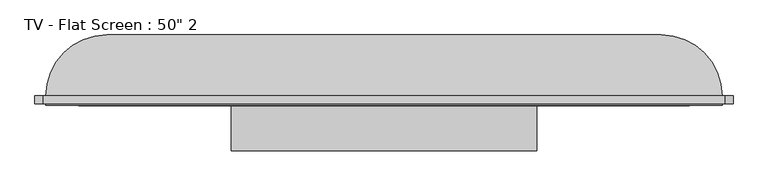
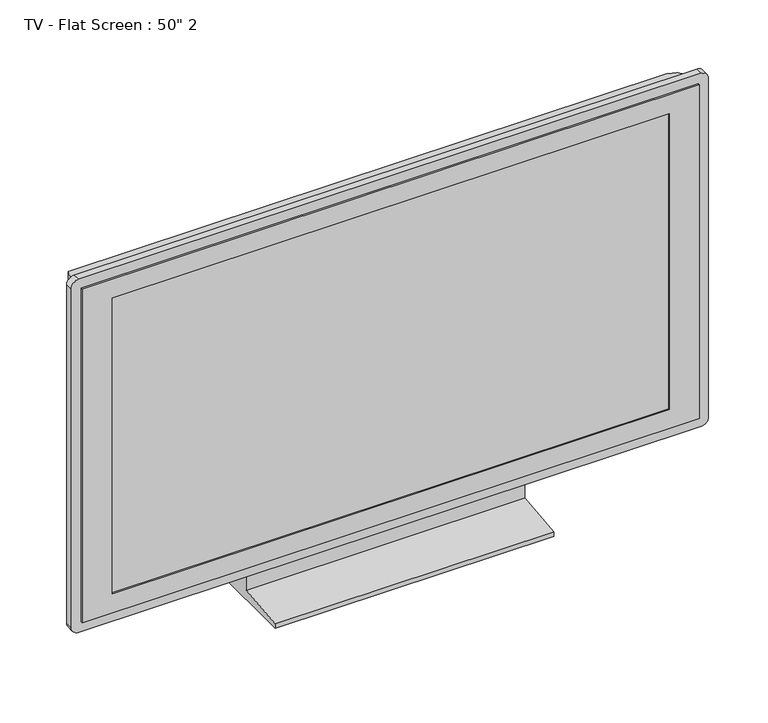
"""IFC4 building model written with IfcOpenShell, lengths in millimetres: furniture geometry."""

from ifc_helpers import new_model, si_unit, point, frame, frame_2d, origin, place, context, project, spatial, polyline, circle_curve, ellipse_curve, trimmed, segment, composite_curve, outline, extrude, faceted_brep, source, transform, mapped, element, save
from ifc_brep_helpers import plane_surface, cylinder_surface, advanced_brep


def furniture_0b81fedb(model_context):
    return source(origin(), model_context, "Body", "SolidModel", [
        advanced_brep(
        [(-617.3827737, -51.4613764, 80.0), (609.4937454, -51.4613764, 80.0), (609.4937454, -51.4613764, 782.6751733), (-617.3827737, -51.4613764, 782.6751733), (499.4937454, 58.5386236, 80.0), (-507.3827737, 58.5386236, 80.0), (-507.3827737, 58.5386236, 672.6751733), (499.4937454, 58.5386236, 672.6751733)],
        [
            (0, 1),
            (1, 2),
            (2, 3),
            (3, 0),
            (4, 5),
            (5, 6),
            (6, 7),
            (7, 4),
            (0, 5, circle_curve(frame((-507.3827737, -51.4613764, 80.0), z_axis=(0.0, 0.0, -1.0), x_axis=(-1.0, 0.0, 0.0)), 110.0)),
            (4, 1, circle_curve(frame((499.4937454, -51.4613764, 80.0), z_axis=(0.0, 0.0, -1.0), x_axis=(1.0, 0.0, 0.0)), 110.0)),
            (7, 2, ellipse_curve(frame((499.4937454, -51.4613764, 672.6751733), z_axis=(0.7071067811865475, 0.0, -0.7071067811865475), x_axis=(0.7071067811865474, 0.0, 0.7071067811865476)), 155.5634919, 110.0)),
            (6, 3, ellipse_curve(frame((-507.3827737, -51.4613764, 672.6751733), z_axis=(0.7071067811865475, 0.0, 0.7071067811865475), x_axis=(-0.7071067811865476, 0.0, 0.7071067811865474)), 155.5634919, 110.0)),
        ],
        [
            plane_surface(frame((-617.3827737, -51.4613764, 782.6751733), z_axis=(0.0, -1.0, 0.0), x_axis=(-1.0, 0.0, 0.0))),
            plane_surface(frame((-617.3827737, 58.5386236, 782.6751733), z_axis=(0.0, 1.0, 0.0), x_axis=(1.0, 0.0, 0.0))),
            plane_surface(frame((-617.3827737, -51.4613764, 80.0), z_axis=(0.0, 0.0, -1.0), x_axis=(0.0, 1.0, 0.0))),
            cylinder_surface(frame((499.4937454, -51.4613764, 80.0), z_axis=(0.0, 0.0, 1.0), x_axis=(1.0, 0.0, 0.0)), 110.0),
            cylinder_surface(frame((609.4937454, -51.4613764, 672.6751733), z_axis=(-1.0, 0.0, 0.0), x_axis=(0.0, 0.0, 1.0)), 110.0),
            cylinder_surface(frame((-507.3827737, -51.4613764, 782.6751733), z_axis=(0.0, 0.0, -1.0), x_axis=(-1.0, 0.0, 0.0)), 110.0),
        ],
        [
            (0, [[1, 2, 3, 4]]),
            (1, [[5, 6, 7, 8]]),
            (2, [[-1, 9, -5, 10]]),
            (3, [[11, -2, -10, -8]]),
            (4, [[-11, -7, 12, -3]]),
            (5, [[-12, -6, -9, -4]]),
        ],
    ),
        extrude(outline(composite_curve([segment(polyline([(802.6751733, 614.4937454), (802.6751733, -622.3827737)]), True, "CONTINUOUS"), segment(trimmed(circle_curve(frame_2d((787.6751733, -622.3827737)), 15.0), [point((802.6751733, -622.3827737))], [point((787.6751733, -637.3827737))], False, "CARTESIAN"), True, "CONTINUOUS"), segment(polyline([(787.6751733, -637.3827737), (75.0, -637.3827737)]), True, "CONTINUOUS"), segment(trimmed(circle_curve(frame_2d((75.0, -622.3827737)), 15.0), [point((75.0, -637.3827737))], [point((60.0, -622.3827737))], False, "CARTESIAN"), True, "CONTINUOUS"), segment(polyline([(60.0, -622.3827737), (60.0, 614.4937454)]), True, "CONTINUOUS"), segment(trimmed(circle_curve(frame_2d((75.0, 614.4937454)), 15.0), [point((60.0, 614.4937454))], [point((75.0, 629.4937454))], False, "CARTESIAN"), True, "CONTINUOUS"), segment(polyline([(75.0, 629.4937454), (787.6751733, 629.4937454)]), True, "CONTINUOUS"), segment(trimmed(circle_curve(frame_2d((787.6751733, 614.4937454)), 15.0), [point((787.6751733, 629.4937454))], [point((802.6751733, 614.4937454))], False, "CARTESIAN"), True, "CONTINUOUS")], self_intersect=False), holes=[polyline([(782.6751733, 609.4937454), (80.0, 609.4937454), (80.0, -617.3827737), (782.6751733, -617.3827737), (782.6751733, 609.4937454)])]), frame((0.0, -66.4613764, 0.0), z_axis=(0.0, 1.0, 0.0), x_axis=(0.0, 0.0, 1.0)), (0.0, 0.0, 1.0), 15.0),
        faceted_brep([(609.4937454, -69.4613764, 782.6751733), (-617.3827737, -69.4613764, 782.6751733), (-617.3827737, -69.4613764, 80.0), (609.4937454, -69.4613764, 80.0), (-557.3827737, -69.4613764, 742.6751733), (549.4937454, -69.4613764, 742.6751733), (549.4937454, -69.4613764, 120.0), (-557.3827737, -69.4613764, 120.0), (609.4937454, -51.4613764, 782.6751733), (609.4937454, -51.4613764, 80.0), (-617.3827737, -51.4613764, 80.0), (-617.3827737, -51.4613764, 782.6751733), (-557.3827737, -66.4613764, 742.6751733), (-557.3827737, -66.4613764, 120.0), (549.4937454, -66.4613764, 120.0), (549.4937454, -66.4613764, 742.6751733)], [[[0, 1, 2, 3], [4, 5, 6, 7]], [[8, 9, 10, 11]], [[1, 0, 8, 11]], [[2, 1, 11, 10]], [[3, 2, 10, 9]], [[0, 3, 9, 8]], [[12, 13, 14, 15]], [[12, 15, 5, 4]], [[15, 14, 6, 5]], [[14, 13, 7, 6]], [[13, 12, 4, 7]]]),
        extrude(outline(polyline([(-51.4613764, 80.0), (-1.4613764, 80.0), (48.5386236, 0.0), (-151.4613764, 0.0), (-151.4613764, 10.0), (-51.4613764, 20.0), (-51.4613764, 80.0)])), frame((-280.6636439, 0.0, 0.0), z_axis=(1.0, 0.0, 0.0), x_axis=(0.0, 1.0, 0.0)), (0.0, 0.0, 1.0), 553.4382596),
    ])


if __name__ == "__main__":
    model = new_model("IFC4")
    model_context = context("Model", 3, world=origin())
    ifc_project = project(units=[si_unit("LENGTHUNIT", "METRE", prefix="MILLI")], contexts=[model_context])
    site = spatial("IfcSite", under=ifc_project)
    building = spatial("IfcBuilding", under=site)
    placement = place(None, origin())
    furniture_shape = furniture_0b81fedb(model_context)
    element("IfcFurniture", 1, ObjectType="TV - Flat Screen : 50\" 2", at=placement, inside=building, context=model_context, shape_type="MappedRepresentation", body=[
        mapped(furniture_shape, transform((0.0, 0.0, 0.0), x_axis=(1.0, 0.0, 0.0), y_axis=(0.0, 1.0, 0.0), z_axis=(0.0, 0.0, 1.0))),
    ])
    save(model, "model.ifc")

# Revit data of these elements
# Type "TV - Flat Screen : 50\" 2"
#   SinAng = 0' - 0.0193"
#   L = 3' - 7.57782"
#   H = 2' - 0.51477"
#   Thickness = 0' - 4.33071"
#   Diagonal = 4' - 2"
#   Default Elevation = 3' - 0"
#   CosAng = 0' - 0.03431"
#   Stand [instance default] = yes
# Element 1 (IfcFurniture, "TV - Flat Screen : 50\" 2")
#   Materials on its faces: "TV - Black", "TV - Glass", "TV - Screen"
# Materials
#   "TV - Black": colour RGB 49 49 49, transparency 0
#   "TV - Glass": colour RGB 157 157 157, transparency 0.9
#   "TV - Screen": colour RGB 0 0 0, transparency 0
